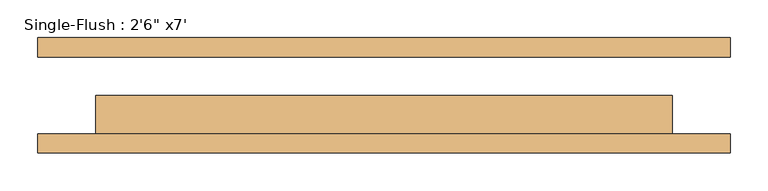
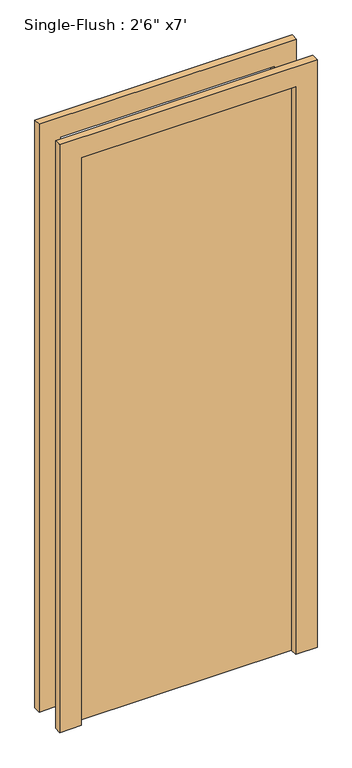
"""IFC4 building model written with IfcOpenShell, lengths in millimetres: door geometry."""

from ifc_helpers import new_model, si_unit, frame, origin, origin_with_axes, place, context, project, spatial, polyline, outline, extrude, source, transform, mapped, element, save


def door_aa9e95e7(model_context):
    return source(origin(), model_context, "Body", "SweptSolid", [
        extrude(outline(polyline([(2209.8, -457.2), (0.0, -457.2), (0.0, -381.0), (2133.6, -381.0), (2133.6, 381.0), (0.0, 381.0), (0.0, 457.2), (2209.8, 457.2), (2209.8, -457.2)])), frame((0.0, -76.2, 0.0), z_axis=(0.0, 1.0, 0.0), x_axis=(0.0, 0.0, 1.0)), (0.0, 0.0, 1.0), 25.4),
        extrude(outline(polyline([(2209.8, 457.2), (2209.8, -457.2), (0.0, -457.2), (0.0, -381.0), (2133.6, -381.0), (2133.6, 381.0), (0.0, 381.0), (0.0, 457.2), (2209.8, 457.2)])), frame((0.0, 50.8, 0.0), z_axis=(0.0, 1.0, 0.0), x_axis=(0.0, 0.0, 1.0)), (0.0, 0.0, 1.0), 25.4),
        extrude(outline(polyline([(381.0, 0.0), (381.0, -50.8), (-381.0, -50.8), (-381.0, 0.0), (381.0, 0.0)])), origin_with_axes(), (0.0, 0.0, 1.0), 2133.6),
    ])


if __name__ == "__main__":
    model = new_model("IFC4")
    model_context = context("Model", 3, world=origin())
    ifc_project = project(units=[si_unit("LENGTHUNIT", "METRE", prefix="MILLI")], contexts=[model_context])
    site = spatial("IfcSite", under=ifc_project)
    building = spatial("IfcBuilding", under=site)
    placement = place(None, origin())
    door_shape = door_aa9e95e7(model_context)
    element("IfcDoor", 1, ObjectType="Single-Flush : 2'6\" x7'", at=placement, inside=building, context=model_context, shape_type="MappedRepresentation", body=[
        mapped(door_shape, transform((0.0, 0.0, 0.0), x_axis=(1.0, 0.0, 0.0), y_axis=(0.0, 1.0, 0.0), z_axis=(0.0, 0.0, 1.0))),
    ])
    save(model, "model.ifc")

# Revit data of these elements
# Type "Single-Flush : 2'6\" x7'"
#   Type Mark = "15"
#   Construction Type Id = "MDOOR"
#   Assembly Code = "C1020"
#   Analytic Construction = "Metal"
#   Thickness = 0' - 2"
#   Heat Transfer Coefficient (U) = 0.651978 BTU/(h·ft²·°F)
#   Height = 7' - 0"
#   Trim Projection Ext = 0' - 1"
#   Trim Projection Int = 0' - 1"
#   Trim Width = 0' - 3"
#   Width = 2' - 6"
#   Define Thermal Properties by = 1
#   Door Material = Door - Panel
#   Frame Material = Door - Frame
#   Visual Light Transmittance = 0
#   Solar Heat Gain Coefficient = 0
#   Function = (empty or 0)
#   Wall Closure = (empty or 0)
# Element 1 (IfcDoor, "Single-Flush : 2'6\" x7'")
#   Materials on its faces: "Door - Frame", "Door - Panel"
# Materials
#   "Door - Panel": class "Wood", colour RGB 210 159 95, transparency 0, Cost = 0
#   "Door - Frame": colour RGB 118 70 51, transparency 0, Cost = 0
